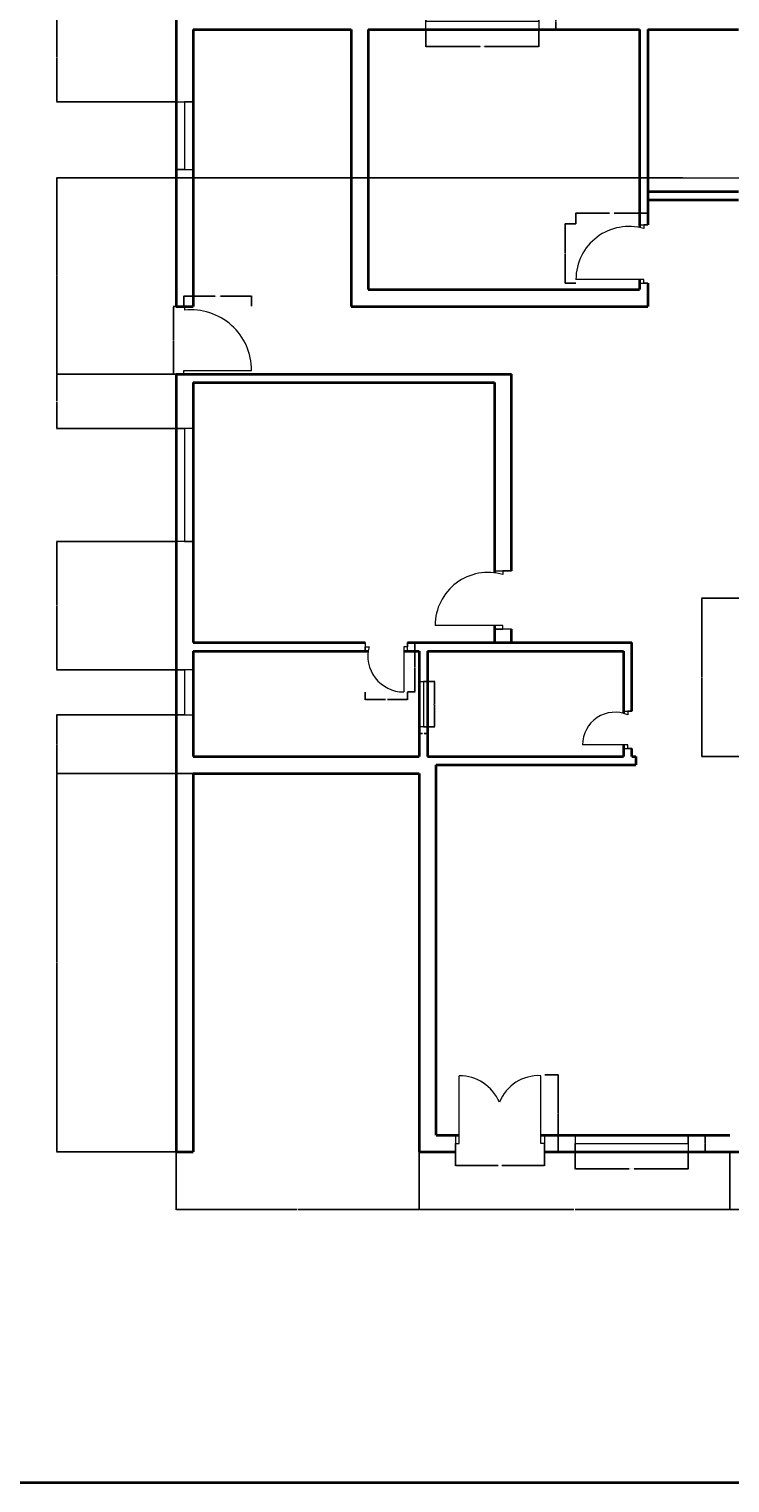
# Model space of a CAD drawing. Units: inches. Extents: x 1152 to 2588, y 1459 to 2618.
# Tile 15 of 17: x 1802 to 2174, y 1459 to 2231. Entities that reach past the tile are written whole.
import ezdxf

# ---------------------------------------------------------------- set-up
doc = ezdxf.new("R2010")
doc.units = ezdxf.units.IN
for name, color, linetype, lineweight in [('A-ANNO-DIMS', 2, 'Continuous', 18), ('A-ANNO-SYMB', 3, 'Continuous', 18), ('A-ANNO-TTLB', 7, 'Continuous', 35), ('A-DOOR', 4, 'Continuous', 18), ('A-GLAZ', 4, 'Continuous', 18), ('A-WALL', 7, 'Continuous', 35)]:
    doc.layers.add(name, color=color, linetype=linetype, lineweight=lineweight)
doc.styles.get("Standard").update_dxf_attribs({"font": 'arial.ttf'})
doc.dimstyles.get("Standard").update_dxf_attribs({"dimtxt": 0.18, "dimasz": 0.18, "dimexe": 0.18, "dimexo": 0.0625, "dimgap": 0.09, "dimtad": 0, "dimtih": 1, "dimtoh": 1, "dimdec": 4, "dimzin": 0, "dimdsep": 46, "dimtxsty": 'Standard', "dimcen": 0.09, "dimadec": 0, "dimazin": 0, "dimtfac": 1, "dimtdec": 4, "dimtofl": 0, "dimtmove": 0, "dimatfit": 3, "dimfxl": 1, "dimtolj": 1, "dimtzin": 0, "dimarcsym": 0})

# ---------------------------------------------------------------- blocks, each defined once
blk = doc.blocks.new('DOOR-DOUBLE-ENTRY')
for p, q in [((2, 4.5), (2, 40.5)), ((45.34, 4.5), (45.34, 40.5)), ((0, 9), (0, 0)), ((47.34, 9), (47.34, 0)), ((0, 0), (0, 4.5)), ((0, 4.5), (2, 4.5)), ((47.34, 4.5), (45.34, 4.5)), ((47.34, 0), (47.34, 4.5))]:
    blk.add_line(p, q)
for centre, radius, start, end in [((2, 17.3), 23.2, 23.30533, 90), ((44.08, 18.16), 22.37, 86.77895, 158.18289)]:
    blk.add_arc(centre, radius, start, end)
blk = doc.blocks.new('DOOR-36-BED-NORTH')
for p, q in [((33.75, 30.96), (38.25, 30.96)), ((38.25, 30.96), (36, 30.96)), ((36, 30.96), (36, 28.96)), ((36, 2), (0, 2)), ((36, 0), (36, 2)), ((33.75, 0), (38.25, 0)), ((38.25, 0), (36, 0))]:
    blk.add_line(p, q)
blk.add_arc((28.09, 2), 28.09, 73.65517, 180)
blk = doc.blocks.new('DOOR-36-BED-WEST')
for p, q in [((31.5, 31), (40.5, 31)), ((40.5, 31), (36, 31)), ((36, 31), (36, 29)), ((36, 2), (0, 2)), ((36, 0), (36, 2)), ((40.5, 0), (31.5, 0)), ((31.5, 0), (36, 0))]:
    blk.add_line(p, q)
blk.add_arc((28.13, 2), 28.13, 73.74705, 180)
blk = doc.blocks.new('DOOR-24-BATH-WEST')
for p, q in [((0, 26.25), (0, 21.75)), ((0, 21.75), (0, 24)), ((0, 24), (2, 24)), ((22.43, 24), (20.43, 24)), ((20.43, 24), (20.43, 0)), ((22.43, 21.75), (22.43, 26.25)), ((22.43, 26.25), (22.43, 24))]:
    blk.add_line(p, q)
blk.add_arc((20.43, 19.08), 19.08, 165.05043, 270)
blk = doc.blocks.new('DOOR-24-BATH-CENTRE')
for p, q in [((21.75, 19.88), (26.25, 19.88)), ((26.25, 19.88), (24, 19.88)), ((24, 19.88), (24, 17.88)), ((24, 2), (0, 2)), ((24, 0), (24, 2)), ((21.75, 0), (26.25, 0)), ((26.25, 0), (24, 0))]:
    blk.add_line(p, q)
blk.add_arc((17.25, 2), 17.25, 66.97541, 180)
blk = doc.blocks.new('DOOR-36-POOJA')
for p, q in [((0.4, 36), (0.4, 34)), ((0, 0), (0, 2)), ((0, 2), (36, 2))]:
    blk.add_line(p, q)
blk.add_arc((3.82, 2), 32.18, 0, 96.10172)
blk = doc.blocks.new('WIN-60-EXT')
for p, q in [((0, 9), (0, 0)), ((60, 4.5), (60, 9)), ((60, 9), (60, 0)), ((0, 0), (0, 4.5)), ((0, 4.5), (60, 4.5))]:
    blk.add_line(p, q)
blk = doc.blocks.new('WIN-36')
for p, q in [((0, 36), (9, 36)), ((9, 36), (4.5, 36)), ((4.5, 36), (4.5, 0)), ((4.5, 0), (0, 0)), ((0, 0), (9, 0))]:
    blk.add_line(p, q)
blk = doc.blocks.new('WIN-60-FRONT')
for p, q in [((0, 9), (0, 0)), ((60, 4.5), (60, 9)), ((60, 9), (60, 0)), ((0, 0), (0, 4.5)), ((0, 4.5), (48, 4.5)), ((48, 4.5), (60, 4.5))]:
    blk.add_line(p, q)
blk = doc.blocks.new('WIN-24-BATH-WEST')
for p, q in [((9, 24), (0, 24)), ((0, 24), (4.5, 24)), ((4.5, 24), (4.5, 0)), ((4.5, 0), (0, 0)), ((0, 0), (9, 0))]:
    blk.add_line(p, q)
blk = doc.blocks.new('WIN-24-INTERIOR')
for p, q in [((0, 24), (4.5, 24)), ((4.5, 24), (2.25, 24)), ((2.25, 24), (2.25, 0)), ((4.5, 0), (0, 0)), ((2.25, 0), (4.5, 0))]:
    blk.add_line(p, q)
blk = doc.blocks.new('WIN-60-BED-NORTH')
for p, q in [((0, 0), (0, 9)), ((0, 9), (0, 4.5)), ((60, 4.5), (60, 9)), ((60, 9), (60, 0)), ((0, 4.5), (60, 4.5))]:
    blk.add_line(p, q)
blk = doc.blocks.new('*D36')
at = {"layer": 'A-ANNO-DIMS', "color": 0, "lineweight": -2, "transparency": 16777216}
for p, q in [((2028.2, 1634.98), (2028.2, 1627.77)), ((2075.53, 1634.98), (2075.53, 1627.77)), ((2028.38, 1627.95), (2050.88, 1627.95)), ((2075.35, 1627.95), (2052.85, 1627.95))]:
    blk.add_line(p, q, dxfattribs=at)
at = {"layer": 'A-ANNO-DIMS', "color": 0, "transparency": 16777216}
for points in [[(2028.38, 1627.98), (2028.38, 1627.92), (2028.2, 1627.95)], [(2075.35, 1627.98), (2075.35, 1627.92), (2075.53, 1627.95)]]:
    blk.add_solid(points, dxfattribs=at)
at = {"layer": 'Defpoints', "color": 0, "transparency": 16777216}
for p in [(2028.2, 1635.05), (2075.53, 1635.05), (2075.53, 1627.95)]:
    blk.add_point(p, dxfattribs=at)
at = {"layer": 'A-ANNO-DIMS', "color": 0, "transparency": 16777216, "insert": (2051.86, 1627.95), "char_height": 0.18, "attachment_point": 5}
blk.add_mtext('\\A1;ENTRY 47 TYP.', dxfattribs=at)
blk = doc.blocks.new('*D37')
at = {"layer": 'A-ANNO-DIMS', "color": 0, "lineweight": -2, "transparency": 16777216}
for p, q in [((2075.6, 1676.09), (2082.81, 1676.09)), ((2082.63, 1675.91), (2082.63, 1655.75)), ((2082.63, 1635.23), (2082.63, 1655.39)), ((2075.6, 1635.05), (2082.81, 1635.05))]:
    blk.add_line(p, q, dxfattribs=at)
at = {"layer": 'A-ANNO-DIMS', "color": 0, "transparency": 16777216}
for points in [[(2082.6, 1675.91), (2082.66, 1675.91), (2082.63, 1676.09)], [(2082.6, 1635.23), (2082.66, 1635.23), (2082.63, 1635.05)]]:
    blk.add_solid(points, dxfattribs=at)
at = {"layer": 'Defpoints', "color": 0, "transparency": 16777216}
for p in [(2075.53, 1676.09), (2082.63, 1676.09), (2075.53, 1635.05)]:
    blk.add_point(p, dxfattribs=at)
at = {"layer": 'A-ANNO-DIMS', "color": 0, "transparency": 16777216, "insert": (2082.63, 1655.57), "char_height": 0.18, "attachment_point": 5}
blk.add_mtext('\\A1;41 TYP.', dxfattribs=at)
blk = doc.blocks.new('*D40')
at = {"layer": 'A-ANNO-DIMS', "color": 0, "lineweight": -2, "transparency": 16777216}
for p, q in [((2092.13, 2127.88), (2092.13, 2133.74)), ((2092.31, 2133.56), (2110.03, 2133.56)), ((2130.2, 2133.56), (2112.49, 2133.56)), ((2130.38, 2127.88), (2130.38, 2133.74))]:
    blk.add_line(p, q, dxfattribs=at)
at = {"layer": 'A-ANNO-DIMS', "color": 0, "transparency": 16777216}
for points in [[(2092.31, 2133.59), (2092.31, 2133.53), (2092.13, 2133.56)], [(2130.2, 2133.59), (2130.2, 2133.53), (2130.38, 2133.56)]]:
    blk.add_solid(points, dxfattribs=at)
at = {"layer": 'Defpoints', "color": 0, "transparency": 16777216}
for p in [(2130.38, 2133.56), (2092.13, 2127.82), (2130.38, 2127.82)]:
    blk.add_point(p, dxfattribs=at)
at = {"layer": 'A-ANNO-DIMS', "color": 0, "transparency": 16777216, "insert": (2111.26, 2133.56), "char_height": 0.18, "attachment_point": 5}
blk.add_mtext('\\A1;BED DOOR 38 TYP.', dxfattribs=at)
blk = doc.blocks.new('*D41')
at = {"layer": 'A-ANNO-DIMS', "color": 0, "lineweight": -2, "transparency": 16777216}
for p, q in [((2092.07, 2127.82), (2086.22, 2127.82)), ((2086.4, 2127.64), (2086.4, 2112.28)), ((2086.4, 2096.55), (2086.4, 2111.92)), ((2092.07, 2096.37), (2086.22, 2096.37))]:
    blk.add_line(p, q, dxfattribs=at)
at = {"layer": 'A-ANNO-DIMS', "color": 0, "transparency": 16777216}
for points in [[(2086.37, 2127.64), (2086.43, 2127.64), (2086.4, 2127.82)], [(2086.37, 2096.55), (2086.43, 2096.55), (2086.4, 2096.37)]]:
    blk.add_solid(points, dxfattribs=at)
at = {"layer": 'Defpoints', "color": 0, "transparency": 16777216}
for p in [(2086.4, 2127.82), (2092.13, 2127.82), (2092.13, 2096.37)]:
    blk.add_point(p, dxfattribs=at)
at = {"layer": 'A-ANNO-DIMS', "color": 0, "transparency": 16777216, "insert": (2086.4, 2112.1), "char_height": 0.18, "attachment_point": 5}
blk.add_mtext('\\A1;31 TYP.', dxfattribs=at)
blk = doc.blocks.new('*D44')
at = {"layer": 'A-ANNO-DIMS', "color": 0, "lineweight": -2, "transparency": 16777216}
for p, q in [((2002.81, 1905.55), (2006.87, 1905.55)), ((2006.69, 1905.37), (2006.69, 1892.6)), ((2006.69, 1879.48), (2006.69, 1892.24)), ((2002.81, 1879.3), (2006.87, 1879.3))]:
    blk.add_line(p, q, dxfattribs=at)
at = {"layer": 'A-ANNO-DIMS', "color": 0, "transparency": 16777216}
for points in [[(2006.66, 1905.37), (2006.72, 1905.37), (2006.69, 1905.55)], [(2006.66, 1879.48), (2006.72, 1879.48), (2006.69, 1879.3)]]:
    blk.add_solid(points, dxfattribs=at)
at = {"layer": 'Defpoints', "color": 0, "transparency": 16777216}
for p in [(2002.75, 1905.55), (2006.69, 1905.55), (2002.75, 1879.3)]:
    blk.add_point(p, dxfattribs=at)
at = {"layer": 'A-ANNO-DIMS', "color": 0, "transparency": 16777216, "insert": (2006.69, 1892.42), "char_height": 0.18, "attachment_point": 5}
blk.add_mtext('\\A1;BATH DOOR 26 TYP.', dxfattribs=at)
blk = doc.blocks.new('*D45')
at = {"layer": 'A-ANNO-DIMS', "color": 0, "lineweight": -2, "transparency": 16777216}
for p, q in [((1980.32, 1879.23), (1980.32, 1875.18)), ((2002.75, 1879.23), (2002.75, 1875.18)), ((1980.5, 1875.36), (1991, 1875.36)), ((2002.57, 1875.36), (1992.06, 1875.36))]:
    blk.add_line(p, q, dxfattribs=at)
at = {"layer": 'A-ANNO-DIMS', "color": 0, "transparency": 16777216}
for points in [[(1980.5, 1875.39), (1980.5, 1875.33), (1980.32, 1875.36)], [(2002.57, 1875.39), (2002.57, 1875.33), (2002.75, 1875.36)]]:
    blk.add_solid(points, dxfattribs=at)
at = {"layer": 'Defpoints', "color": 0, "transparency": 16777216}
for p in [(1980.32, 1879.3), (2002.75, 1879.3), (2002.75, 1875.36)]:
    blk.add_point(p, dxfattribs=at)
at = {"layer": 'A-ANNO-DIMS', "color": 0, "transparency": 16777216, "insert": (1991.53, 1875.36), "char_height": 0.18, "attachment_point": 5}
blk.add_mtext('\\A1;22 TYP.', dxfattribs=at)
blk = doc.blocks.new('*D50')
at = {"layer": 'A-ANNO-DIMS', "color": 0, "lineweight": -2, "transparency": 16777216}
for p, q in [((1883.99, 2084.11), (1883.99, 2089.63)), ((1884.17, 2089.45), (1900.59, 2089.45)), ((1919.81, 2089.45), (1903.38, 2089.45)), ((1919.99, 2084.11), (1919.99, 2089.63))]:
    blk.add_line(p, q, dxfattribs=at)
at = {"layer": 'A-ANNO-DIMS', "color": 0, "transparency": 16777216}
for points in [[(1884.17, 2089.48), (1884.17, 2089.42), (1883.99, 2089.45)], [(1919.81, 2089.48), (1919.81, 2089.42), (1919.99, 2089.45)]]:
    blk.add_solid(points, dxfattribs=at)
at = {"layer": 'Defpoints', "color": 0, "transparency": 16777216}
for p in [(1919.99, 2089.45), (1883.99, 2084.05), (1919.99, 2084.05)]:
    blk.add_point(p, dxfattribs=at)
at = {"layer": 'A-ANNO-DIMS', "color": 0, "transparency": 16777216, "insert": (1901.99, 2089.45), "char_height": 0.18, "attachment_point": 5}
blk.add_mtext('\\A1;POOJA DOOR 36 TYP.', dxfattribs=at)
blk = doc.blocks.new('*D51')
at = {"layer": 'A-ANNO-DIMS', "color": 0, "lineweight": -2, "transparency": 16777216}
for p, q in [((1883.92, 2084.05), (1878.41, 2084.05)), ((1878.59, 2083.87), (1878.59, 2066.23)), ((1878.59, 2048.23), (1878.59, 2065.86)), ((1883.92, 2048.05), (1878.41, 2048.05))]:
    blk.add_line(p, q, dxfattribs=at)
at = {"layer": 'A-ANNO-DIMS', "color": 0, "transparency": 16777216}
for points in [[(1878.56, 2083.87), (1878.62, 2083.87), (1878.59, 2084.05)], [(1878.56, 2048.23), (1878.62, 2048.23), (1878.59, 2048.05)]]:
    blk.add_solid(points, dxfattribs=at)
at = {"layer": 'Defpoints', "color": 0, "transparency": 16777216}
for p in [(1878.59, 2084.05), (1883.99, 2084.05), (1883.99, 2048.05)]:
    blk.add_point(p, dxfattribs=at)
at = {"layer": 'A-ANNO-DIMS', "color": 0, "transparency": 16777216, "insert": (1878.59, 2066.05), "char_height": 0.18, "attachment_point": 5}
blk.add_mtext('\\A1;36 TYP.', dxfattribs=at)
blk = doc.blocks.new('*D54')
at = {"layer": 'A-ANNO-DIMS', "color": 0, "lineweight": -2, "transparency": 16777216}
for p, q in [((2091.7, 1634.98), (2091.7, 1625.87)), ((2151.7, 1634.98), (2151.7, 1625.87)), ((2091.88, 1626.05), (2120.4, 1626.05)), ((2151.52, 1626.05), (2123.01, 1626.05))]:
    blk.add_line(p, q, dxfattribs=at)
at = {"layer": 'A-ANNO-DIMS', "color": 0, "transparency": 16777216}
for points in [[(2091.88, 1626.08), (2091.88, 1626.02), (2091.7, 1626.05)], [(2151.52, 1626.08), (2151.52, 1626.02), (2151.7, 1626.05)]]:
    blk.add_solid(points, dxfattribs=at)
at = {"layer": 'Defpoints', "color": 0, "transparency": 16777216}
for p in [(2091.7, 1635.05), (2151.7, 1635.05), (2151.7, 1626.05)]:
    blk.add_point(p, dxfattribs=at)
at = {"layer": 'A-ANNO-DIMS', "color": 0, "transparency": 16777216, "insert": (2121.7, 1626.05), "char_height": 0.18, "attachment_point": 5}
blk.add_mtext('\\A1;FRONT WIN. 60 TYP.', dxfattribs=at)
blk = doc.blocks.new('*D55')
at = {"layer": 'A-ANNO-DIMS', "color": 0, "lineweight": -2, "transparency": 16777216}
for p, q in [((2151.77, 1644.05), (2160.88, 1644.05)), ((2160.7, 1643.87), (2160.7, 1639.73)), ((2160.7, 1635.23), (2160.7, 1639.36)), ((2151.77, 1635.05), (2160.88, 1635.05))]:
    blk.add_line(p, q, dxfattribs=at)
at = {"layer": 'A-ANNO-DIMS', "color": 0, "transparency": 16777216}
for points in [[(2160.67, 1643.87), (2160.73, 1643.87), (2160.7, 1644.05)], [(2160.67, 1635.23), (2160.73, 1635.23), (2160.7, 1635.05)]]:
    blk.add_solid(points, dxfattribs=at)
at = {"layer": 'Defpoints', "color": 0, "transparency": 16777216}
for p in [(2151.7, 1644.05), (2160.7, 1644.05), (2151.7, 1635.05)]:
    blk.add_point(p, dxfattribs=at)
at = {"layer": 'A-ANNO-DIMS', "color": 0, "transparency": 16777216, "insert": (2160.7, 1639.55), "char_height": 0.18, "attachment_point": 5}
blk.add_mtext('\\A1;9 TYP.', dxfattribs=at)
blk = doc.blocks.new('*D60')
at = {"layer": 'A-ANNO-DIMS', "color": 0, "lineweight": -2, "transparency": 16777216}
for p, q in [((2013.45, 1884.86), (2017.16, 1884.86)), ((2016.98, 1884.68), (2016.98, 1873.04)), ((2016.98, 1861.04), (2016.98, 1872.68)), ((2013.45, 1860.86), (2017.16, 1860.86))]:
    blk.add_line(p, q, dxfattribs=at)
at = {"layer": 'A-ANNO-DIMS', "color": 0, "transparency": 16777216}
for points in [[(2016.95, 1884.68), (2017.01, 1884.68), (2016.98, 1884.86)], [(2016.95, 1861.04), (2017.01, 1861.04), (2016.98, 1860.86)]]:
    blk.add_solid(points, dxfattribs=at)
at = {"layer": 'Defpoints', "color": 0, "transparency": 16777216}
for p in [(2013.38, 1884.86), (2016.98, 1884.86), (2013.38, 1860.86)]:
    blk.add_point(p, dxfattribs=at)
at = {"layer": 'A-ANNO-DIMS', "color": 0, "transparency": 16777216, "insert": (2016.98, 1872.86), "char_height": 0.18, "attachment_point": 5}
blk.add_mtext('\\A1;WIN. 24 TYP.', dxfattribs=at)
blk = doc.blocks.new('*D61')
at = {"layer": 'A-ANNO-DIMS', "color": 0, "lineweight": -2, "transparency": 16777216}
for p, q in [((2008.88, 1860.8), (2008.88, 1857.08)), ((2013.38, 1860.8), (2013.38, 1857.08)), ((2009.06, 1857.26), (2010.68, 1857.26)), ((2013.2, 1857.26), (2011.59, 1857.26))]:
    blk.add_line(p, q, dxfattribs=at)
at = {"layer": 'A-ANNO-DIMS', "color": 0, "transparency": 16777216}
for points in [[(2009.06, 1857.29), (2009.06, 1857.23), (2008.88, 1857.26)], [(2013.2, 1857.29), (2013.2, 1857.23), (2013.38, 1857.26)]]:
    blk.add_solid(points, dxfattribs=at)
at = {"layer": 'Defpoints', "color": 0, "transparency": 16777216}
for p in [(2008.88, 1860.86), (2013.38, 1860.86), (2013.38, 1857.26)]:
    blk.add_point(p, dxfattribs=at)
at = {"layer": 'A-ANNO-DIMS', "color": 0, "transparency": 16777216, "insert": (2011.13, 1857.26), "char_height": 0.18, "attachment_point": 5}
blk.add_mtext('\\A1;5 TYP.', dxfattribs=at)
blk = doc.blocks.new('*D64')
at = {"layer": 'A-ANNO-DIMS', "color": 0, "lineweight": -2, "transparency": 16777216}
for p, q in [((2012.39, 2230.98), (2012.39, 2221.87)), ((2072.39, 2230.98), (2072.39, 2221.87)), ((2012.57, 2222.05), (2041.26, 2222.05)), ((2072.21, 2222.05), (2043.53, 2222.05))]:
    blk.add_line(p, q, dxfattribs=at)
at = {"layer": 'A-ANNO-DIMS', "color": 0, "transparency": 16777216}
for points in [[(2012.57, 2222.08), (2012.57, 2222.02), (2012.39, 2222.05)], [(2072.21, 2222.08), (2072.21, 2222.02), (2072.39, 2222.05)]]:
    blk.add_solid(points, dxfattribs=at)
at = {"layer": 'Defpoints', "color": 0, "transparency": 16777216}
for p in [(2012.39, 2231.05), (2072.39, 2231.05), (2072.39, 2222.05)]:
    blk.add_point(p, dxfattribs=at)
at = {"layer": 'A-ANNO-DIMS', "color": 0, "transparency": 16777216, "insert": (2042.39, 2222.05), "char_height": 0.18, "attachment_point": 5}
blk.add_mtext('\\A1;BED WIN. 60 TYP.', dxfattribs=at)
blk = doc.blocks.new('*D65')
at = {"layer": 'A-ANNO-DIMS', "color": 0, "lineweight": -2, "transparency": 16777216}
for p, q in [((2072.46, 2240.05), (2081.57, 2240.05)), ((2081.39, 2239.87), (2081.39, 2235.73)), ((2072.46, 2231.05), (2081.57, 2231.05)), ((2081.39, 2231.23), (2081.39, 2235.36))]:
    blk.add_line(p, q, dxfattribs=at)
at = {"layer": 'A-ANNO-DIMS', "color": 0, "transparency": 16777216}
for points in [[(2081.36, 2239.87), (2081.42, 2239.87), (2081.39, 2240.05)], [(2081.36, 2231.23), (2081.42, 2231.23), (2081.39, 2231.05)]]:
    blk.add_solid(points, dxfattribs=at)
at = {"layer": 'Defpoints', "color": 0, "transparency": 16777216}
for p in [(2072.39, 2240.05), (2081.39, 2240.05), (2072.39, 2231.05)]:
    blk.add_point(p, dxfattribs=at)
at = {"layer": 'A-ANNO-DIMS', "color": 0, "transparency": 16777216, "insert": (2081.39, 2235.55), "char_height": 0.18, "attachment_point": 5}
blk.add_mtext('\\A1;9 TYP.', dxfattribs=at)
blk = doc.blocks.new('*D67')
at = {"layer": 'A-ANNO-DIMS', "color": 0, "lineweight": -2, "transparency": 16777216}
for p, q in [((2179.93, 1929.05), (2158.72, 1929.05)), ((2158.9, 1928.87), (2158.9, 1887.23)), ((2158.9, 1845.23), (2158.9, 1886.86)), ((2179.93, 1845.05), (2158.72, 1845.05))]:
    blk.add_line(p, q, dxfattribs=at)
at = {"layer": 'A-ANNO-DIMS', "color": 0, "transparency": 16777216}
for points in [[(2158.87, 1928.87), (2158.93, 1928.87), (2158.9, 1929.05)], [(2158.87, 1845.23), (2158.93, 1845.23), (2158.9, 1845.05)]]:
    blk.add_solid(points, dxfattribs=at)
at = {"layer": 'Defpoints', "color": 0, "transparency": 16777216}
for p in [(2158.9, 1929.05), (2179.99, 1929.05), (2179.99, 1845.05)]:
    blk.add_point(p, dxfattribs=at)
at = {"layer": 'A-ANNO-DIMS', "color": 0, "transparency": 16777216, "insert": (2158.9, 1887.05), "char_height": 0.18, "attachment_point": 5}
blk.add_mtext('\\A1;84 TYP.', dxfattribs=at)
blk = doc.blocks.new('*D79')
at = {"layer": 'A-ANNO-DIMS', "color": 0, "lineweight": -2, "transparency": 16777216}
for p, q in [((1888.82, 1836.05), (1816.39, 1836.05)), ((1816.57, 1835.87), (1816.57, 1735.73)), ((1816.57, 1635.23), (1816.57, 1735.36)), ((1879.82, 1635.05), (1816.39, 1635.05))]:
    blk.add_line(p, q, dxfattribs=at)
at = {"layer": 'A-ANNO-DIMS', "color": 0, "transparency": 16777216}
for points in [[(1816.54, 1835.87), (1816.6, 1835.87), (1816.57, 1836.05)], [(1816.54, 1635.23), (1816.6, 1635.23), (1816.57, 1635.05)]]:
    blk.add_solid(points, dxfattribs=at)
at = {"layer": 'Defpoints', "color": 0, "transparency": 16777216}
for p in [(1816.57, 1836.05), (1888.88, 1836.05), (1879.88, 1635.05)]:
    blk.add_point(p, dxfattribs=at)
at = {"layer": 'A-ANNO-DIMS', "color": 0, "transparency": 16777216, "insert": (1816.57, 1735.55), "char_height": 0.18, "attachment_point": 5}
blk.add_mtext('\\A1;201', dxfattribs=at)
blk = doc.blocks.new('*D80')
at = {"layer": 'A-ANNO-DIMS', "color": 0, "lineweight": -2, "transparency": 16777216}
for p, q in [((1879.82, 1867.13), (1816.39, 1867.13)), ((1816.57, 1866.95), (1816.57, 1851.77)), ((1816.57, 1836.23), (1816.57, 1851.41)), ((1888.82, 1836.05), (1816.39, 1836.05))]:
    blk.add_line(p, q, dxfattribs=at)
at = {"layer": 'A-ANNO-DIMS', "color": 0, "transparency": 16777216}
for points in [[(1816.54, 1866.95), (1816.6, 1866.95), (1816.57, 1867.13)], [(1816.54, 1836.23), (1816.6, 1836.23), (1816.57, 1836.05)]]:
    blk.add_solid(points, dxfattribs=at)
at = {"layer": 'Defpoints', "color": 0, "transparency": 16777216}
for p in [(1816.57, 1867.13), (1879.88, 1867.13), (1888.88, 1836.05)]:
    blk.add_point(p, dxfattribs=at)
at = {"layer": 'A-ANNO-DIMS', "color": 0, "transparency": 16777216, "insert": (1816.57, 1851.59), "char_height": 0.18, "attachment_point": 5}
blk.add_mtext('\\A1;31.086', dxfattribs=at)
blk = doc.blocks.new('*D81')
at = {"layer": 'A-ANNO-DIMS', "color": 0, "lineweight": -2, "transparency": 16777216}
for p, q in [((1879.82, 1959.21), (1816.39, 1959.21)), ((1816.57, 1959.03), (1816.57, 1925.35)), ((1816.57, 1891.31), (1816.57, 1924.99)), ((1879.82, 1891.13), (1816.39, 1891.13))]:
    blk.add_line(p, q, dxfattribs=at)
at = {"layer": 'A-ANNO-DIMS', "color": 0, "transparency": 16777216}
for points in [[(1816.54, 1959.03), (1816.6, 1959.03), (1816.57, 1959.21)], [(1816.54, 1891.31), (1816.6, 1891.31), (1816.57, 1891.13)]]:
    blk.add_solid(points, dxfattribs=at)
at = {"layer": 'Defpoints', "color": 0, "transparency": 16777216}
for p in [(1816.57, 1959.21), (1879.88, 1959.21), (1879.88, 1891.13)]:
    blk.add_point(p, dxfattribs=at)
at = {"layer": 'A-ANNO-DIMS', "color": 0, "transparency": 16777216, "insert": (1816.57, 1925.17), "char_height": 0.18, "attachment_point": 5}
blk.add_mtext('\\A1;68.08', dxfattribs=at)
blk = doc.blocks.new('*D82')
at = {"layer": 'A-ANNO-DIMS', "color": 0, "lineweight": -2, "transparency": 16777216}
for p, q in [((1879.82, 2048.05), (1816.39, 2048.05)), ((1816.57, 2047.87), (1816.57, 2033.81)), ((1816.57, 2019.39), (1816.57, 2033.44)), ((1879.82, 2019.21), (1816.39, 2019.21))]:
    blk.add_line(p, q, dxfattribs=at)
at = {"layer": 'A-ANNO-DIMS', "color": 0, "transparency": 16777216}
for points in [[(1816.54, 2047.87), (1816.6, 2047.87), (1816.57, 2048.05)], [(1816.54, 2019.39), (1816.6, 2019.39), (1816.57, 2019.21)]]:
    blk.add_solid(points, dxfattribs=at)
at = {"layer": 'Defpoints', "color": 0, "transparency": 16777216}
for p in [(1816.57, 2048.05), (1879.88, 2048.05), (1879.88, 2019.21)]:
    blk.add_point(p, dxfattribs=at)
at = {"layer": 'A-ANNO-DIMS', "color": 0, "transparency": 16777216, "insert": (1816.57, 2033.63), "char_height": 0.18, "attachment_point": 5}
blk.add_mtext('\\A1;28.84', dxfattribs=at)
blk = doc.blocks.new('*D83')
at = {"layer": 'A-ANNO-DIMS', "color": 0, "lineweight": -2, "transparency": 16777216}
for p, q in [((1847.11, 2152.33), (1816.39, 2152.33)), ((1816.57, 2152.15), (1816.57, 2100.37)), ((1816.57, 2048.23), (1816.57, 2100.01)), ((1879.82, 2048.05), (1816.39, 2048.05))]:
    blk.add_line(p, q, dxfattribs=at)
at = {"layer": 'A-ANNO-DIMS', "color": 0, "transparency": 16777216}
for points in [[(1816.54, 2152.15), (1816.6, 2152.15), (1816.57, 2152.33)], [(1816.54, 2048.23), (1816.6, 2048.23), (1816.57, 2048.05)]]:
    blk.add_solid(points, dxfattribs=at)
at = {"layer": 'Defpoints', "color": 0, "transparency": 16777216}
for p in [(1816.57, 2152.33), (1847.17, 2152.33), (1879.88, 2048.05)]:
    blk.add_point(p, dxfattribs=at)
at = {"layer": 'A-ANNO-DIMS', "color": 0, "transparency": 16777216, "insert": (1816.57, 2100.19), "char_height": 0.18, "attachment_point": 5}
blk.add_mtext('\\A1;104.29', dxfattribs=at)
blk = doc.blocks.new('*D84')
at = {"layer": 'A-ANNO-DIMS', "color": 0, "lineweight": -2, "transparency": 16777216}
for p, q in [((1879.82, 2240.05), (1816.39, 2240.05)), ((1816.57, 2239.87), (1816.57, 2216.58)), ((1816.57, 2192.93), (1816.57, 2216.22)), ((1879.82, 2192.75), (1816.39, 2192.75))]:
    blk.add_line(p, q, dxfattribs=at)
at = {"layer": 'A-ANNO-DIMS', "color": 0, "transparency": 16777216}
for points in [[(1816.54, 2239.87), (1816.6, 2239.87), (1816.57, 2240.05)], [(1816.54, 2192.93), (1816.6, 2192.93), (1816.57, 2192.75)]]:
    blk.add_solid(points, dxfattribs=at)
at = {"layer": 'Defpoints', "color": 0, "transparency": 16777216}
for p in [(1816.57, 2240.05), (1879.88, 2240.05), (1879.88, 2192.75)]:
    blk.add_point(p, dxfattribs=at)
at = {"layer": 'A-ANNO-DIMS', "color": 0, "transparency": 16777216, "insert": (1816.57, 2216.4), "char_height": 0.18, "attachment_point": 5}
blk.add_mtext('\\A1;47.3', dxfattribs=at)
blk = doc.blocks.new('*D85')
at = {"layer": 'A-ANNO-DIMS', "color": 0, "lineweight": -2, "transparency": 16777216}
for p, q in [((1879.88, 1634.98), (1879.88, 1604.27)), ((2008.88, 1634.98), (2008.88, 1604.27)), ((1880.06, 1604.45), (1944.1, 1604.45)), ((2008.7, 1604.45), (1944.66, 1604.45))]:
    blk.add_line(p, q, dxfattribs=at)
at = {"layer": 'A-ANNO-DIMS', "color": 0, "transparency": 16777216}
for points in [[(1880.06, 1604.48), (1880.06, 1604.42), (1879.88, 1604.45)], [(2008.7, 1604.48), (2008.7, 1604.42), (2008.88, 1604.45)]]:
    blk.add_solid(points, dxfattribs=at)
at = {"layer": 'Defpoints', "color": 0, "transparency": 16777216}
for p in [(1879.88, 1635.05), (2008.88, 1635.05), (2008.88, 1604.45)]:
    blk.add_point(p, dxfattribs=at)
at = {"layer": 'A-ANNO-DIMS', "color": 0, "transparency": 16777216, "insert": (1944.38, 1604.45), "char_height": 0.18, "attachment_point": 5}
blk.add_mtext('\\A1;129', dxfattribs=at)
blk = doc.blocks.new('*D86')
at = {"layer": 'A-ANNO-DIMS', "color": 0, "lineweight": -2, "transparency": 16777216}
for p, q in [((2008.88, 1634.98), (2008.88, 1604.27)), ((2173.88, 1634.98), (2173.88, 1604.27)), ((2009.06, 1604.45), (2091.1, 1604.45)), ((2173.7, 1604.45), (2091.67, 1604.45))]:
    blk.add_line(p, q, dxfattribs=at)
at = {"layer": 'A-ANNO-DIMS', "color": 0, "transparency": 16777216}
for points in [[(2009.06, 1604.48), (2009.06, 1604.42), (2008.88, 1604.45)], [(2173.7, 1604.48), (2173.7, 1604.42), (2173.88, 1604.45)]]:
    blk.add_solid(points, dxfattribs=at)
at = {"layer": 'Defpoints', "color": 0, "transparency": 16777216}
for p in [(2008.88, 1635.05), (2173.88, 1635.05), (2173.88, 1604.45)]:
    blk.add_point(p, dxfattribs=at)
at = {"layer": 'A-ANNO-DIMS', "color": 0, "transparency": 16777216, "insert": (2091.38, 1604.45), "char_height": 0.18, "attachment_point": 5}
blk.add_mtext('\\A1;165', dxfattribs=at)
blk = doc.blocks.new('*D87')
at = {"layer": 'A-ANNO-DIMS', "color": 0, "lineweight": -2, "transparency": 16777216}
for p, q in [((2173.88, 1634.98), (2173.88, 1604.27)), ((2339.88, 1634.98), (2339.88, 1604.27)), ((2174.06, 1604.45), (2256.6, 1604.45)), ((2339.7, 1604.45), (2257.16, 1604.45))]:
    blk.add_line(p, q, dxfattribs=at)
at = {"layer": 'A-ANNO-DIMS', "color": 0, "transparency": 16777216}
for points in [[(2174.06, 1604.48), (2174.06, 1604.42), (2173.88, 1604.45)], [(2339.7, 1604.48), (2339.7, 1604.42), (2339.88, 1604.45)]]:
    blk.add_solid(points, dxfattribs=at)
at = {"layer": 'Defpoints', "color": 0, "transparency": 16777216}
for p in [(2173.88, 1635.05), (2339.88, 1635.05), (2339.88, 1604.45)]:
    blk.add_point(p, dxfattribs=at)
at = {"layer": 'A-ANNO-DIMS', "color": 0, "transparency": 16777216, "insert": (2256.88, 1604.45), "char_height": 0.18, "attachment_point": 5}
blk.add_mtext('\\A1;166', dxfattribs=at)

msp = doc.modelspace()

# ---------------------------------------------------------------- linework, layer by layer
at = {"layer": 'A-ANNO-SYMB'}
for p, q in [((2148.8526, 2152.3313), (1847.169, 2152.3313)), ((1847.169, 2152.3313), (2386.5775, 2152.3313))]:
    msp.add_line(p, q, dxfattribs=at)
at = {"layer": 'A-ANNO-TTLB'}
msp.add_lwpolyline([(1152.3215, 2617.6685), (2587.6987, 2617.6685), (2587.6987, 1459.3148), (1152.3215, 1459.3148)], close=True, dxfattribs=at)
at = {"layer": 'A-WALL'}
for p, q in [((1879.8841, 2240.0458), (1879.8841, 2084.0458)), ((1888.8841, 2231.0458), (1972.8841, 2231.0458)), ((1888.8841, 2231.0458), (1888.8841, 2084.0458)), ((1972.8841, 2231.0458), (1972.8841, 2084.0458)), ((1981.8841, 2231.0458), (2125.8841, 2231.0458)), ((1981.8841, 2231.0458), (1981.8841, 2093.0458)), ((2125.8841, 2231.0458), (2125.8841, 2125.8914)), ((2130.3841, 2231.0458), (2178.3841, 2231.0458)), ((2130.3841, 2231.0458), (2130.3841, 2127.3313)), ((2130.3841, 2145.0458), (2178.3841, 2145.0458)), ((2130.3841, 2140.5458), (2178.3841, 2140.5458)), ((1981.8841, 2093.0458), (2125.8841, 2093.0458)), ((2125.8841, 2098.3728), (2125.8841, 2093.0458)), ((2130.3841, 2096.3728), (2130.3841, 2084.0458)), ((1879.8841, 2084.0458), (1888.8841, 2084.0458)), ((1972.8841, 2084.0458), (2130.3841, 2084.0458)), ((1879.8841, 2048.0458), (1879.8841, 1635.0458)), ((1879.8841, 2048.0458), (2057.8841, 2048.0458)), ((2057.8841, 1943.6503), (2057.8841, 2048.0458)), ((1888.8841, 2043.5458), (1888.8841, 1905.5458)), ((1888.8841, 2043.5458), (2048.8841, 2043.5458)), ((1888.8841, 2043.5458), (2048.8841, 2043.5458)), ((2048.8841, 2043.5458), (2048.8841, 1942.5716)), ((2048.8841, 1914.6468), (2048.8841, 1905.5458)), ((2057.8841, 1905.5458), (2057.8841, 1912.6468)), ((1888.8841, 1905.5458), (1980.3181, 1905.5458)), ((1888.8841, 1901.0458), (1888.8841, 1845.0458)), ((1888.8841, 1901.0458), (1981.8604, 1901.0458)), ((2000.7507, 1901.0458), (2008.8841, 1901.0458)), ((2002.7507, 1905.5458), (2121.8841, 1905.5458)), ((2008.8841, 1901.0458), (2008.8841, 1845.0458)), ((2013.3841, 1901.0458), (2013.3841, 1845.0458)), ((2013.3841, 1901.0458), (2117.3841, 1901.0458)), ((2048.8841, 1905.5458), (2057.8841, 1905.5458)), ((2117.3841, 1901.0458), (2117.3841, 1867.9483)), ((2121.8841, 1869.1706), (2121.8841, 1905.5458)), ((1888.8841, 1845.0458), (2008.8841, 1845.0458)), ((2013.3841, 1845.0458), (2117.3841, 1845.0458)), ((2117.3841, 1851.2927), (2117.3841, 1845.0458)), ((2121.8841, 1845.0458), (2121.8841, 1849.2927)), ((2121.8841, 1845.0458), (2123.9904, 1845.0458)), ((2123.9904, 1845.0458), (2123.9904, 1840.5831)), ((2017.8841, 1836.0458), (2017.8841, 1840.5831)), ((2017.8841, 1840.5831), (2123.9904, 1840.5831)), ((1888.8841, 1836.0458), (1888.8841, 1635.0458)), ((1888.8841, 1836.0458), (2008.8841, 1836.0458)), ((2008.8841, 1836.0458), (2008.8841, 1635.0458)), ((2017.8841, 1644.0458), (2017.8841, 1836.0458)), ((2017.8841, 1644.0458), (2030.1953, 1644.0458)), ((2073.5339, 1644.0458), (2173.8841, 1644.0458)), ((1879.8841, 1635.0458), (1888.8841, 1635.0458)), ((2008.8841, 1635.0458), (2028.1953, 1635.0458)), ((2008.8841, 1635.0458), (2017.8841, 1635.0458)), ((2075.5339, 1635.0458), (2339.8841, 1635.0458))]:
    msp.add_line(p, q, dxfattribs=at)

# ---------------------------------------------------------------- block references
at = {"layer": 'A-DOOR'}
for name, p in [('DOOR-36-BED-NORTH', (2092.1346, 2096.373)), ('DOOR-36-POOJA', (1883.9876, 2048.046)), ('DOOR-36-BED-WEST', (2017.3846, 1912.647)), ('DOOR-24-BATH-WEST', (1980.3186, 1879.296)), ('DOOR-24-BATH-CENTRE', (2095.6346, 1849.293)), ('DOOR-DOUBLE-ENTRY', (2028.1956, 1635.046))]:
    msp.add_blockref(name, p, dxfattribs=at)
at = {"layer": 'A-GLAZ'}
for name, p in [('WIN-60-BED-NORTH', (2012.3946, 2231.046)), ('WIN-36', (1879.8846, 2156.749)), ('WIN-24-BATH-WEST', (1879.8846, 1867.132)), ('WIN-24-INTERIOR', (2008.8846, 1860.858)), ('WIN-60-FRONT', (2091.7036, 1635.046))]:
    msp.add_blockref(name, p, dxfattribs=at)
at = {"layer": 'A-GLAZ', "rotation": 270.0000000000007}
msp.add_blockref('WIN-60-EXT', (1879.8843, 2019.2078), dxfattribs=at)

# ---------------------------------------------------------------- dimensions: what is measured, and where the dimension line sits
at = {"layer": 'A-ANNO-DIMS'}
for base, p1, p2, override, picture, middle in [((1816.569, 2240.0458), (1879.8841, 2192.7491), (1879.8841, 2240.0458), {"dimdec": 1, "dimlfac": 1, "dimrnd": 0, "dimzin": 0, "dimdsep": 46, "dimlunit": 2}, '*D84', (1816.569, 2216.3975)), ((1816.569, 2152.3313), (1879.8841, 2048.0458), (1847.169, 2152.3313), {"dimdec": 2, "dimlfac": 1, "dimrnd": 0, "dimzin": 0, "dimdsep": 46, "dimlunit": 2}, '*D83', (1816.569, 2100.1886)), ((1816.569, 2048.0458), (1879.8841, 2019.2077), (1879.8841, 2048.0458), {"dimdec": 2, "dimlfac": 1, "dimrnd": 0, "dimzin": 0, "dimdsep": 46, "dimlunit": 2}, '*D82', (1816.569, 2033.6268)), ((1816.569, 1959.2077), (1879.8841, 1891.1319), (1879.8841, 1959.2077), {"dimdec": 2, "dimlfac": 1, "dimrnd": 0, "dimzin": 0, "dimdsep": 46, "dimlunit": 2}, '*D81', (1816.569, 1925.1698)), ((1816.569, 1867.1319), (1888.8841, 1836.0458), (1879.8841, 1867.1319), {"dimdec": 3, "dimlfac": 1, "dimrnd": 0, "dimzin": 0, "dimdsep": 46, "dimlunit": 2}, '*D80', (1816.569, 1851.5889)), ((1816.569, 1836.0458), (1879.8841, 1635.0458), (1888.8841, 1836.0458), {"dimdec": 0, "dimlfac": 1, "dimrnd": 0, "dimzin": 0, "dimdsep": 46, "dimlunit": 2}, '*D79', (1816.569, 1735.5458))]:
    dim = msp.add_linear_dim(base=base, p1=p1, p2=p2, angle=90, dimstyle='Standard', override=override, dxfattribs=at)
    dim.commit()
    dim.dimension.update_dxf_attribs({"geometry": picture, "text_midpoint": middle})
for base, p1, p2, text, picture, middle in [((2081.3947, 2240.0458), (2072.3947, 2231.0458), (2072.3947, 2240.0458), '<> TYP.', '*D65', (2081.3947, 2235.5458)), ((2086.3966, 2127.8218), (2092.1341, 2096.3728), (2092.1341, 2127.8218), '<> TYP.', '*D41', (2086.3966, 2112.0973)), ((1878.5872, 2084.0458), (1883.9872, 2048.0458), (1883.9872, 2084.0458), '<> TYP.', '*D51', (1878.5872, 2066.0458)), ((2158.9012, 1929.0458), (2179.9911, 1845.0458), (2179.9911, 1929.0458), '<> TYP.', '*D67', (2158.9012, 1887.0458)), ((2006.6882, 1905.5458), (2002.7507, 1879.2958), (2002.7507, 1905.5458), 'BATH DOOR <> TYP.', '*D44', (2006.6882, 1892.4208)), ((2016.9841, 1884.8579), (2013.3841, 1860.8579), (2013.3841, 1884.8579), 'WIN. <> TYP.', '*D60', (2016.9841, 1872.8579)), ((2082.6347, 1676.0856), (2075.5339, 1635.0458), (2075.5339, 1676.0856), '<> TYP.', '*D37', (2082.6347, 1655.5657)), ((2160.7035, 1644.0458), (2151.7035, 1635.0458), (2151.7035, 1644.0458), '<> TYP.', '*D55', (2160.7035, 1639.5458))]:
    dim = msp.add_linear_dim(base=base, p1=p1, p2=p2, angle=90, text=text, dimstyle='Standard', override={"dimdec": 0, "dimlfac": 1, "dimrnd": 0, "dimzin": 0, "dimdsep": 46, "dimlunit": 2}, dxfattribs=at)
    dim.commit()
    dim.dimension.update_dxf_attribs({"geometry": picture, "text_midpoint": middle})
for base, p1, p2, text, picture, middle in [((2072.3947, 2222.0458), (2012.3947, 2231.0458), (2072.3947, 2231.0458), 'BED WIN. <> TYP.', '*D64', (2042.3947, 2222.0458)), ((2130.3841, 2133.5593), (2092.1341, 2127.8218), (2130.3841, 2127.8218), 'BED DOOR <> TYP.', '*D40', (2111.2591, 2133.5593)), ((1919.9872, 2089.4458), (1883.9872, 2084.0458), (1919.9872, 2084.0458), 'POOJA DOOR <> TYP.', '*D50', (1901.9872, 2089.4458)), ((2002.7507, 1875.3583), (1980.3181, 1879.2958), (2002.7507, 1879.2958), '<> TYP.', '*D45', (1991.5344, 1875.3583)), ((2013.3841041472, 1857.2578999201), (2008.8841041472, 1860.8578999201), (2013.3841041472, 1860.8578999201), '<> TYP.', '*D61', (2011.1341041472, 1857.2578999201)), ((2075.5339, 1627.945), (2028.1953, 1635.0458), (2075.5339, 1635.0458), 'ENTRY <> TYP.', '*D36', (2051.8646, 1627.945)), ((2151.7035, 1626.0458), (2091.7035, 1635.0458), (2151.7035, 1635.0458), 'FRONT WIN. <> TYP.', '*D54', (2121.7035, 1626.0458))]:
    dim = msp.add_linear_dim(base=base, p1=p1, p2=p2, text=text, dimstyle='Standard', override={"dimdec": 0, "dimlfac": 1, "dimrnd": 0, "dimzin": 0, "dimdsep": 46, "dimlunit": 2}, dxfattribs=at)
    dim.commit()
    dim.dimension.update_dxf_attribs({"geometry": picture, "text_midpoint": middle})
for base, p1, p2, picture, middle in [((2008.8841, 1604.4458), (1879.8841, 1635.0458), (2008.8841, 1635.0458), '*D85', (1944.3841, 1604.4458)), ((2173.8841, 1604.4458), (2008.8841, 1635.0458), (2173.8841, 1635.0458), '*D86', (2091.3841, 1604.4458)), ((2339.8841, 1604.4458), (2173.8841, 1635.0458), (2339.8841, 1635.0458), '*D87', (2256.8841, 1604.4458))]:
    dim = msp.add_linear_dim(base=base, p1=p1, p2=p2, dimstyle='Standard', override={"dimdec": 0, "dimlfac": 1, "dimrnd": 0, "dimzin": 0, "dimdsep": 46, "dimlunit": 2}, dxfattribs=at)
    dim.commit()
    dim.dimension.update_dxf_attribs({"geometry": picture, "text_midpoint": middle})

doc.saveas('drawing.dxf')
